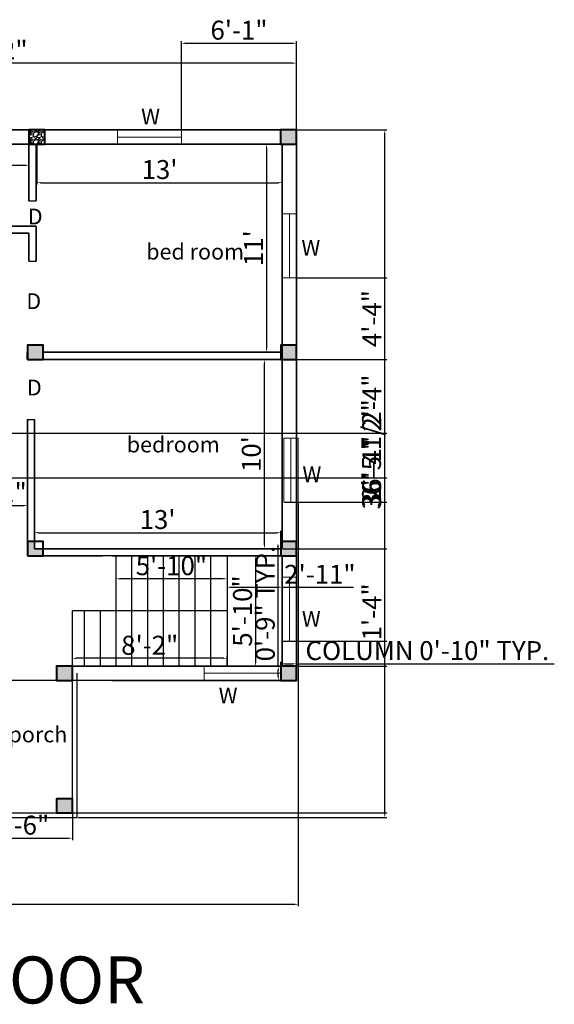
# Model space of a CAD drawing. Units: inches. Extents: x 1989 to 3287, y 1752 to 2384.
# Tile 5 of 5: x 2948 to 3287, y 1752 to 2377. Entities that reach past the tile are written whole.
import ezdxf

# ---------------------------------------------------------------- set-up
doc = ezdxf.new("R2010")
doc.units = ezdxf.units.IN
for name, color, linetype, lineweight in [('A-ANNO-DIMS', 2, 'Continuous', 18), ('A-ANNO-TEXT', 7, 'Continuous', 18), ('A-AREA-IDEN', 7, 'Continuous', 18), ('A-COLS', 1, 'Continuous', 40), ('A-COLS-PATT', 8, 'Continuous', 13), ('A-DOOR', 3, 'Continuous', 25), ('A-FLOR-EDGE', 7, 'Continuous', 25), ('A-FLOR-STRS', 7, 'Continuous', 25), ('A-GLAZ', 4, 'Continuous', 18), ('A-WALL', 7, 'Continuous', 35)]:
    doc.layers.add(name, color=color, linetype=linetype, lineweight=lineweight)
doc.styles.get("Standard").update_dxf_attribs({"font": 'arial.ttf'})
doc.dimstyles.new('ISO-25', dxfattribs={"dimtxt": 12, "dimasz": 2.5, "dimexe": 1.25, "dimexo": 0.625, "dimtad": 1, "dimdec": 0, "dimlunit": 4, "dimtxsty": 'Standard', "dimcen": 2.5, "dimadec": 0, "dimazin": 0, "dimtfac": 1, "dimtdec": 0, "dimtmove": 0, "dimatfit": 3, "dimfxl": 1, "dimarcsym": 0})

# ---------------------------------------------------------------- blocks, each defined once
blk = doc.blocks.new('*D19')
at = {"layer": 'A-ANNO-DIMS', "color": 0, "lineweight": -2, "transparency": 16777216}
for p, q in [((2915.71, 1873.05), (2915.71, 1856.37)), ((2981.21, 1873.05), (2981.21, 1856.37)), ((2918.21, 1857.62), (2978.71, 1857.62))]:
    blk.add_line(p, q, dxfattribs=at)
at = {"layer": 'A-ANNO-DIMS', "color": 0, "transparency": 16777216}
for points in [[(2918.21, 1858.04), (2918.21, 1857.2), (2915.71, 1857.62)], [(2978.71, 1858.04), (2978.71, 1857.2), (2981.21, 1857.62)]]:
    blk.add_solid(points, dxfattribs=at)
at = {"layer": 'Defpoints', "color": 0, "transparency": 16777216}
for p in [(2915.71, 1873.68), (2981.21, 1873.68), (2981.21, 1857.62)]:
    blk.add_point(p, dxfattribs=at)
at = {"layer": 'A-ANNO-DIMS', "color": 0, "transparency": 16777216, "insert": (2948.46, 1864.37), "char_height": 12, "attachment_point": 5}
blk.add_mtext('5\'-6"', dxfattribs=at)
blk = doc.blocks.new('*D20')
at = {"layer": 'A-ANNO-DIMS', "color": 0, "lineweight": -2, "transparency": 16777216}
for p, q in [((3079.21, 2028.42), (3079.21, 2015.48)), ((3114.21, 2028.42), (3114.21, 2015.48)), ((3081.71, 2016.73), (3111.71, 2016.73)), ((3114.21, 2016.73), (3159.39, 2016.73))]:
    blk.add_line(p, q, dxfattribs=at)
at = {"layer": 'A-ANNO-DIMS', "color": 0, "transparency": 16777216}
for points in [[(3081.71, 2017.15), (3081.71, 2016.31), (3079.21, 2016.73)], [(3111.71, 2017.15), (3111.71, 2016.31), (3114.21, 2016.73)]]:
    blk.add_solid(points, dxfattribs=at)
at = {"layer": 'Defpoints', "color": 0, "transparency": 16777216}
for p in [(3079.21, 2029.04), (3114.21, 2029.04), (3114.21, 2016.73)]:
    blk.add_point(p, dxfattribs=at)
at = {"layer": 'A-ANNO-DIMS', "color": 0, "transparency": 16777216, "insert": (3138.05, 2023.38), "char_height": 12, "attachment_point": 5}
blk.add_mtext('2\'-11"', dxfattribs=at)
blk = doc.blocks.new('*D21')
at = {"layer": 'A-ANNO-DIMS', "color": 0, "lineweight": -2, "transparency": 16777216}
for p, q in [((3079.83, 2036.68), (3098.58, 2036.68)), ((3097.33, 2034.18), (3097.33, 1969.18)), ((3079.83, 1966.68), (3098.58, 1966.68))]:
    blk.add_line(p, q, dxfattribs=at)
at = {"layer": 'A-ANNO-DIMS', "color": 0, "transparency": 16777216}
for points in [[(3096.91, 2034.18), (3097.75, 2034.18), (3097.33, 2036.68)], [(3096.91, 1969.18), (3097.75, 1969.18), (3097.33, 1966.68)]]:
    blk.add_solid(points, dxfattribs=at)
at = {"layer": 'Defpoints', "color": 0, "transparency": 16777216}
for p in [(3079.21, 2036.68), (3079.21, 1966.68), (3097.33, 1966.68)]:
    blk.add_point(p, dxfattribs=at)
at = {"layer": 'A-ANNO-DIMS', "color": 0, "transparency": 16777216, "insert": (3090.58, 2001.68), "char_height": 12, "attachment_point": 5, "rotation": 90}
blk.add_mtext('5\'-10"', dxfattribs=at)
blk = doc.blocks.new('*D22')
at = {"layer": 'A-ANNO-DIMS', "color": 0, "lineweight": -2, "transparency": 16777216}
for p, q in [((3008.71, 2036.05), (3008.71, 2020.84)), ((3079.21, 2036.05), (3079.21, 2020.84)), ((3076.71, 2022.09), (3011.21, 2022.09))]:
    blk.add_line(p, q, dxfattribs=at)
at = {"layer": 'A-ANNO-DIMS', "color": 0, "transparency": 16777216}
for points in [[(3011.21, 2022.5), (3011.21, 2021.67), (3008.71, 2022.09)], [(3076.71, 2022.5), (3076.71, 2021.67), (3079.21, 2022.09)]]:
    blk.add_solid(points, dxfattribs=at)
at = {"layer": 'Defpoints', "color": 0, "transparency": 16777216}
for p in [(3008.71, 2036.68), (3079.21, 2036.68), (3008.71, 2022.09)]:
    blk.add_point(p, dxfattribs=at)
at = {"layer": 'A-ANNO-DIMS', "color": 0, "transparency": 16777216, "insert": (3043.96, 2028.84), "char_height": 12, "attachment_point": 5}
blk.add_mtext('5\'-10"', dxfattribs=at)
blk = doc.blocks.new('*D23')
at = {"layer": 'A-ANNO-DIMS', "color": 0, "lineweight": -2, "transparency": 16777216}
for p, q in [((2981.21, 1967.3), (2981.21, 1972.92)), ((3079.21, 1967.3), (3079.21, 1972.92)), ((3076.71, 1971.67), (2983.71, 1971.67))]:
    blk.add_line(p, q, dxfattribs=at)
at = {"layer": 'A-ANNO-DIMS', "color": 0, "transparency": 16777216}
for points in [[(2983.71, 1972.08), (2983.71, 1971.25), (2981.21, 1971.67)], [(3076.71, 1972.08), (3076.71, 1971.25), (3079.21, 1971.67)]]:
    blk.add_solid(points, dxfattribs=at)
at = {"layer": 'Defpoints', "color": 0, "transparency": 16777216}
for p in [(2981.21, 1971.67), (2981.21, 1966.68), (3079.21, 1966.68)]:
    blk.add_point(p, dxfattribs=at)
at = {"layer": 'A-ANNO-DIMS', "color": 0, "transparency": 16777216, "insert": (3030.21, 1978.42), "char_height": 12, "attachment_point": 5}
blk.add_mtext('8\'-2"', dxfattribs=at)
blk = doc.blocks.new('*D27')
at = {"layer": 'A-ANNO-DIMS', "color": 0, "lineweight": -2, "transparency": 16777216}
for p, q in [((2737.21, 2307.3), (2737.21, 2350.26)), ((3120.71, 2349.01), (2739.71, 2349.01)), ((3123.21, 2307.3), (3123.21, 2350.26))]:
    blk.add_line(p, q, dxfattribs=at)
at = {"layer": 'A-ANNO-DIMS', "color": 0, "transparency": 16777216}
for points in [[(2739.71, 2349.43), (2739.71, 2348.6), (2737.21, 2349.01)], [(3120.71, 2349.43), (3120.71, 2348.6), (3123.21, 2349.01)]]:
    blk.add_solid(points, dxfattribs=at)
at = {"layer": 'Defpoints', "color": 0, "transparency": 16777216}
for p in [(2737.21, 2349.01), (2737.21, 2306.68), (3123.21, 2306.68)]:
    blk.add_point(p, dxfattribs=at)
at = {"layer": 'A-ANNO-DIMS', "color": 0, "transparency": 16777216, "insert": (2930.21, 2355.77), "char_height": 12, "attachment_point": 5}
blk.add_mtext('32\'-2"', dxfattribs=at)
blk = doc.blocks.new('*D28')
at = {"layer": 'A-ANNO-DIMS', "color": 0, "lineweight": -2, "transparency": 16777216}
for p, q in [((3113.58, 2297.68), (3102.92, 2297.68)), ((3104.17, 2295.18), (3104.17, 2168.18)), ((3113.58, 2165.68), (3102.92, 2165.68))]:
    blk.add_line(p, q, dxfattribs=at)
at = {"layer": 'A-ANNO-DIMS', "color": 0, "transparency": 16777216}
for points in [[(3103.76, 2295.18), (3104.59, 2295.18), (3104.17, 2297.68)], [(3103.76, 2168.18), (3104.59, 2168.18), (3104.17, 2165.68)]]:
    blk.add_solid(points, dxfattribs=at)
at = {"layer": 'Defpoints', "color": 0, "transparency": 16777216}
for p in [(3114.21, 2297.68), (3104.17, 2165.68), (3114.21, 2165.68)]:
    blk.add_point(p, dxfattribs=at)
at = {"layer": 'A-ANNO-DIMS', "color": 0, "transparency": 16777216, "insert": (3097.52, 2231.68), "char_height": 12, "attachment_point": 5, "rotation": 90}
blk.add_mtext("11'", dxfattribs=at)
blk = doc.blocks.new('*D29')
at = {"layer": 'A-ANNO-DIMS', "color": 0, "lineweight": -2, "transparency": 16777216}
for p, q in [((2958.71, 2297.05), (2958.71, 2271.98)), ((3114.21, 2297.05), (3114.21, 2271.98)), ((2961.21, 2273.23), (3111.71, 2273.23))]:
    blk.add_line(p, q, dxfattribs=at)
at = {"layer": 'A-ANNO-DIMS', "color": 0, "transparency": 16777216}
for points in [[(2961.21, 2273.65), (2961.21, 2272.82), (2958.71, 2273.23)], [(3111.71, 2273.65), (3111.71, 2272.82), (3114.21, 2273.23)]]:
    blk.add_solid(points, dxfattribs=at)
at = {"layer": 'Defpoints', "color": 0, "transparency": 16777216}
for p in [(2958.71, 2297.68), (3114.21, 2297.68), (3114.21, 2273.23)]:
    blk.add_point(p, dxfattribs=at)
at = {"layer": 'A-ANNO-DIMS', "color": 0, "transparency": 16777216, "insert": (3036.46, 2279.99), "char_height": 12, "attachment_point": 5}
blk.add_mtext("13'", dxfattribs=at)
blk = doc.blocks.new('*D39')
at = {"layer": 'A-ANNO-DIMS', "color": 0, "lineweight": -2, "transparency": 16777216}
for p, q in [((2883.71, 2297.05), (2883.71, 2282.99)), ((2953.71, 2297.05), (2953.71, 2282.99)), ((2886.21, 2284.24), (2951.21, 2284.24))]:
    blk.add_line(p, q, dxfattribs=at)
at = {"layer": 'A-ANNO-DIMS', "color": 0, "transparency": 16777216}
for points in [[(2886.21, 2284.65), (2886.21, 2283.82), (2883.71, 2284.24)], [(2951.21, 2284.65), (2951.21, 2283.82), (2953.71, 2284.24)]]:
    blk.add_solid(points, dxfattribs=at)
at = {"layer": 'Defpoints', "color": 0, "transparency": 16777216}
for p in [(2883.71, 2297.68), (2953.71, 2297.68), (2953.71, 2284.24)]:
    blk.add_point(p, dxfattribs=at)
at = {"layer": 'A-ANNO-DIMS', "color": 0, "transparency": 16777216, "insert": (2918.71, 2290.99), "char_height": 12, "attachment_point": 5}
blk.add_mtext('5\'-10"', dxfattribs=at)
blk = doc.blocks.new('*D42')
at = {"layer": 'A-ANNO-DIMS', "color": 0, "lineweight": -2, "transparency": 16777216}
for p, q in [((3113.58, 2161.18), (3101.67, 2161.18)), ((3102.92, 2043.68), (3102.92, 2158.68)), ((3113.58, 2041.18), (3101.67, 2041.18))]:
    blk.add_line(p, q, dxfattribs=at)
at = {"layer": 'A-ANNO-DIMS', "color": 0, "transparency": 16777216}
for points in [[(3102.51, 2158.68), (3103.34, 2158.68), (3102.92, 2161.18)], [(3102.51, 2043.68), (3103.34, 2043.68), (3102.92, 2041.18)]]:
    blk.add_solid(points, dxfattribs=at)
at = {"layer": 'Defpoints', "color": 0, "transparency": 16777216}
for p in [(3102.92, 2161.18), (3114.21, 2161.18), (3114.21, 2041.18)]:
    blk.add_point(p, dxfattribs=at)
at = {"layer": 'A-ANNO-DIMS', "color": 0, "transparency": 16777216, "insert": (3096.17, 2101.18), "char_height": 12, "attachment_point": 5, "rotation": 90}
blk.add_mtext("10'", dxfattribs=at)
blk = doc.blocks.new('*D43')
at = {"layer": 'A-ANNO-DIMS', "color": 0, "lineweight": -2, "transparency": 16777216}
for p, q in [((2957.21, 2041.8), (2957.21, 2052.59)), ((2959.71, 2051.34), (3110.71, 2051.34)), ((3113.21, 2041.8), (3113.21, 2052.59))]:
    blk.add_line(p, q, dxfattribs=at)
at = {"layer": 'A-ANNO-DIMS', "color": 0, "transparency": 16777216}
for points in [[(2959.71, 2051.76), (2959.71, 2050.92), (2957.21, 2051.34)], [(3110.71, 2051.76), (3110.71, 2050.92), (3113.21, 2051.34)]]:
    blk.add_solid(points, dxfattribs=at)
at = {"layer": 'Defpoints', "color": 0, "transparency": 16777216}
for p in [(3113.21, 2051.34), (2957.21, 2041.18), (3113.21, 2041.18)]:
    blk.add_point(p, dxfattribs=at)
at = {"layer": 'A-ANNO-DIMS', "color": 0, "transparency": 16777216, "insert": (3035.21, 2058.1), "char_height": 12, "attachment_point": 5}
blk.add_mtext("13'", dxfattribs=at)
blk = doc.blocks.new('*D47')
at = {"layer": 'A-ANNO-DIMS', "color": 0, "lineweight": -2, "transparency": 16777216}
for p, q in [((2915.71, 2037.3), (2915.71, 2069.77)), ((2918.21, 2068.52), (2950.21, 2068.52)), ((2952.71, 2037.3), (2952.71, 2069.77))]:
    blk.add_line(p, q, dxfattribs=at)
at = {"layer": 'A-ANNO-DIMS', "color": 0, "transparency": 16777216}
for points in [[(2918.21, 2068.93), (2918.21, 2068.1), (2915.71, 2068.52)], [(2950.21, 2068.93), (2950.21, 2068.1), (2952.71, 2068.52)]]:
    blk.add_solid(points, dxfattribs=at)
at = {"layer": 'Defpoints', "color": 0, "transparency": 16777216}
for p in [(2952.71, 2068.52), (2915.71, 2036.68), (2952.71, 2036.68)]:
    blk.add_point(p, dxfattribs=at)
at = {"layer": 'A-ANNO-DIMS', "color": 0, "transparency": 16777216, "insert": (2934.21, 2075.27), "char_height": 12, "attachment_point": 5}
blk.add_mtext('3\'-1"', dxfattribs=at)
blk = doc.blocks.new('WIN-EXT-STANDARD')
blk.add_line((4.5, 0), (4.5, 40.55))
blk.add_lwpolyline([(0, 40.55), (9, 40.55), (9, 0), (0, 0)], close=True)
blk = doc.blocks.new('WIN-STAIR-FRONT')
blk.add_line((0, 4.5), (48.49, 4.5))
blk.add_lwpolyline([(48.49, 9), (0, 9), (0, 0), (48.49, 0)], close=True)
blk = doc.blocks.new('COLUMN-10X9')
blk.add_lwpolyline([(0, 0), (10, 0), (10, 9), (0, 9)], close=True)
blk = doc.blocks.new('*D61')
at = {"layer": 'A-ANNO-DIMS', "color": 0, "lineweight": -2, "transparency": 16777216}
for p, q in [((3113.2, 1967.3), (3113.2, 1969.43)), ((3115.7, 1968.18), (3120.7, 1968.18)), ((3123.2, 1967.3), (3123.2, 1969.43)), ((3123.2, 1968.18), (3286.59, 1968.18))]:
    blk.add_line(p, q, dxfattribs=at)
at = {"layer": 'A-ANNO-DIMS', "color": 0, "transparency": 16777216}
for points in [[(3115.7, 1968.6), (3115.7, 1967.76), (3113.2, 1968.18)], [(3120.7, 1968.6), (3120.7, 1967.76), (3123.2, 1968.18)]]:
    blk.add_solid(points, dxfattribs=at)
at = {"layer": 'Defpoints', "color": 0, "transparency": 16777216}
for p in [(3113.2, 1966.68), (3123.2, 1968.18), (3123.2, 1966.68)]:
    blk.add_point(p, dxfattribs=at)
at = {"layer": 'A-ANNO-DIMS', "color": 0, "transparency": 16777216, "insert": (3206.14, 1975.01), "char_height": 12, "attachment_point": 5}
blk.add_mtext('COLUMN 0\'-10" TYP.', dxfattribs=at)
blk = doc.blocks.new('*D62')
at = {"layer": 'A-ANNO-DIMS', "color": 0, "lineweight": -2, "transparency": 16777216}
for p, q in [((3111.7, 1966.68), (3111.7, 2043.58)), ((3112.58, 1966.68), (3110.45, 1966.68)), ((3111.7, 1960.18), (3111.7, 1964.18)), ((3112.58, 1957.68), (3110.45, 1957.68))]:
    blk.add_line(p, q, dxfattribs=at)
at = {"layer": 'A-ANNO-DIMS', "color": 0, "transparency": 16777216}
for points in [[(3111.29, 1964.18), (3112.12, 1964.18), (3111.7, 1966.68)], [(3111.29, 1960.18), (3112.12, 1960.18), (3111.7, 1957.68)]]:
    blk.add_solid(points, dxfattribs=at)
at = {"layer": 'Defpoints', "color": 0, "transparency": 16777216}
for p in [(3111.7, 1966.68), (3113.2, 1966.68), (3113.2, 1957.68)]:
    blk.add_point(p, dxfattribs=at)
at = {"layer": 'A-ANNO-DIMS', "color": 0, "transparency": 16777216, "insert": (3104.95, 2006.38), "char_height": 12, "attachment_point": 5, "rotation": 90}
blk.add_mtext('0\'-9" TYP.', dxfattribs=at)
blk = doc.blocks.new('*D64')
at = {"layer": 'A-ANNO-DIMS', "color": 0, "lineweight": -2, "transparency": 16777216}
for p, q in [((2521.26, 2306.68), (3180.41, 2306.68)), ((3179.16, 1876.18), (3179.16, 2304.18)), ((2379.26, 1873.68), (3180.41, 1873.68))]:
    blk.add_line(p, q, dxfattribs=at)
at = {"layer": 'A-ANNO-DIMS', "color": 0, "transparency": 16777216}
for points in [[(3178.74, 2304.18), (3179.58, 2304.18), (3179.16, 2306.68)], [(3178.74, 1876.18), (3179.58, 1876.18), (3179.16, 1873.68)]]:
    blk.add_solid(points, dxfattribs=at)
at = {"layer": 'Defpoints', "color": 0, "transparency": 16777216}
for p in [(2520.64, 2306.68), (3179.16, 2306.68), (2378.64, 1873.68)]:
    blk.add_point(p, dxfattribs=at)
at = {"layer": 'A-ANNO-DIMS', "color": 0, "transparency": 16777216, "insert": (3172.4, 2090.18), "char_height": 12, "attachment_point": 5, "rotation": 90}
blk.add_mtext('36\'-1"', dxfattribs=at)
blk = doc.blocks.new('*D65')
at = {"layer": 'A-ANNO-DIMS', "color": 0, "lineweight": -2, "transparency": 16777216}
for p, q in [((3124.21, 2069.99), (3124.21, 1814.48)), ((2671.06, 1892.56), (2671.06, 1814.48)), ((2673.56, 1815.73), (3121.71, 1815.73))]:
    blk.add_line(p, q, dxfattribs=at)
at = {"layer": 'A-ANNO-DIMS', "color": 0, "transparency": 16777216}
for points in [[(2673.56, 1816.15), (2673.56, 1815.31), (2671.06, 1815.73)], [(3121.71, 1816.15), (3121.71, 1815.31), (3124.21, 1815.73)]]:
    blk.add_solid(points, dxfattribs=at)
at = {"layer": 'Defpoints', "color": 0, "transparency": 16777216}
for p in [(3124.21, 2070.62), (2671.06, 1893.19), (3124.21, 1815.73)]:
    blk.add_point(p, dxfattribs=at)
at = {"layer": 'A-ANNO-DIMS', "color": 0, "transparency": 16777216, "insert": (2897.63, 1822.49), "char_height": 12, "attachment_point": 5}
blk.add_mtext('37\'-9"', dxfattribs=at)
blk = doc.blocks.new('*D66')
at = {"layer": 'A-ANNO-DIMS', "color": 0, "lineweight": -2, "transparency": 16777216}
for p, q in [((3123.83, 2306.68), (3180.41, 2306.68)), ((3179.16, 1873.18), (3179.16, 2304.18)), ((2984.83, 1870.68), (3180.41, 1870.68))]:
    blk.add_line(p, q, dxfattribs=at)
at = {"layer": 'A-ANNO-DIMS', "color": 0, "transparency": 16777216}
for points in [[(3178.74, 2304.18), (3179.58, 2304.18), (3179.16, 2306.68)], [(3178.74, 1873.18), (3179.58, 1873.18), (3179.16, 1870.68)]]:
    blk.add_solid(points, dxfattribs=at)
at = {"layer": 'Defpoints', "color": 0, "transparency": 16777216}
for p in [(3123.21, 2306.68), (3179.16, 2306.68), (2984.21, 1870.68)]:
    blk.add_point(p, dxfattribs=at)
at = {"layer": 'A-ANNO-DIMS', "color": 0, "transparency": 16777216, "insert": (3172.4, 2088.68), "char_height": 12, "attachment_point": 5, "rotation": 90}
blk.add_mtext('36\'-4"', dxfattribs=at)
blk = doc.blocks.new('*D69')
at = {"layer": 'A-ANNO-DIMS', "color": 0, "lineweight": -2, "transparency": 16777216}
for p, q in [((3123.83, 2212.94), (3180.41, 2212.94)), ((3179.16, 2163.68), (3179.16, 2210.44)), ((3123.83, 2161.18), (3180.41, 2161.18))]:
    blk.add_line(p, q, dxfattribs=at)
at = {"layer": 'A-ANNO-DIMS', "color": 0, "transparency": 16777216}
for points in [[(3178.74, 2210.44), (3179.58, 2210.44), (3179.16, 2212.94)], [(3178.74, 2163.68), (3179.58, 2163.68), (3179.16, 2161.18)]]:
    blk.add_solid(points, dxfattribs=at)
at = {"layer": 'Defpoints', "color": 0, "transparency": 16777216}
for p in [(3123.21, 2212.94), (3179.16, 2212.94), (3123.21, 2161.18)]:
    blk.add_point(p, dxfattribs=at)
at = {"layer": 'A-ANNO-DIMS', "color": 0, "transparency": 16777216, "insert": (3172.53, 2187.06), "char_height": 12, "attachment_point": 5, "rotation": 90}
blk.add_mtext('4\'-4"', dxfattribs=at)
blk = doc.blocks.new('*D70')
at = {"layer": 'A-ANNO-DIMS', "color": 0, "lineweight": -2, "transparency": 16777216}
for p, q in [((3179.16, 2070.62), (3179.16, 2134.43)), ((3115.83, 2070.62), (3180.41, 2070.62)), ((3179.16, 2043.68), (3179.16, 2068.12)), ((3114.83, 2041.18), (3180.41, 2041.18))]:
    blk.add_line(p, q, dxfattribs=at)
at = {"layer": 'A-ANNO-DIMS', "color": 0, "transparency": 16777216}
for points in [[(3178.74, 2068.12), (3179.58, 2068.12), (3179.16, 2070.62)], [(3178.74, 2043.68), (3179.58, 2043.68), (3179.16, 2041.18)]]:
    blk.add_solid(points, dxfattribs=at)
at = {"layer": 'Defpoints', "color": 0, "transparency": 16777216}
for p in [(3115.21, 2070.62), (3179.16, 2070.62), (3114.21, 2041.18)]:
    blk.add_point(p, dxfattribs=at)
at = {"layer": 'A-ANNO-DIMS', "color": 0, "transparency": 16777216, "insert": (3172.33, 2103.78), "char_height": 12, "attachment_point": 5, "rotation": 90}
blk.add_mtext('2\'-5 1/2"', dxfattribs=at)
blk = doc.blocks.new('*D71')
at = {"layer": 'A-ANNO-DIMS', "color": 0, "lineweight": -2, "transparency": 16777216}
for p, q in [((3179.16, 1982.63), (3179.16, 2017.15)), ((3114.83, 1982.63), (3180.41, 1982.63)), ((3179.16, 1969.18), (3179.16, 1980.13)), ((3114.83, 1966.68), (3180.41, 1966.68))]:
    blk.add_line(p, q, dxfattribs=at)
at = {"layer": 'A-ANNO-DIMS', "color": 0, "transparency": 16777216}
for points in [[(3178.74, 1980.13), (3179.58, 1980.13), (3179.16, 1982.63)], [(3178.74, 1969.18), (3179.58, 1969.18), (3179.16, 1966.68)]]:
    blk.add_solid(points, dxfattribs=at)
at = {"layer": 'Defpoints', "color": 0, "transparency": 16777216}
for p in [(3114.21, 1982.63), (3179.16, 1982.63), (3114.21, 1966.68)]:
    blk.add_point(p, dxfattribs=at)
at = {"layer": 'A-ANNO-DIMS', "color": 0, "transparency": 16777216, "insert": (3172.51, 2001.14), "char_height": 12, "attachment_point": 5, "rotation": 90}
blk.add_mtext('1\'-4"', dxfattribs=at)
blk = doc.blocks.new('*D72')
at = {"layer": 'A-ANNO-DIMS', "color": 0, "lineweight": -2, "transparency": 16777216}
for p, q in [((3050.36, 2307.3), (3050.36, 2362.88)), ((3052.86, 2361.63), (3120.71, 2361.63)), ((3123.21, 2307.3), (3123.21, 2362.88))]:
    blk.add_line(p, q, dxfattribs=at)
at = {"layer": 'A-ANNO-DIMS', "color": 0, "transparency": 16777216}
for points in [[(3052.86, 2362.05), (3052.86, 2361.21), (3050.36, 2361.63)], [(3120.71, 2362.05), (3120.71, 2361.21), (3123.21, 2361.63)]]:
    blk.add_solid(points, dxfattribs=at)
at = {"layer": 'Defpoints', "color": 0, "transparency": 16777216}
for p in [(3123.21, 2361.63), (3050.36, 2306.68), (3123.21, 2306.68)]:
    blk.add_point(p, dxfattribs=at)
at = {"layer": 'A-ANNO-DIMS', "color": 0, "transparency": 16777216, "insert": (3086.79, 2368.38), "char_height": 12, "attachment_point": 5}
blk.add_mtext('6\'-1"', dxfattribs=at)
blk = doc.blocks.new('*D74')
at = {"layer": 'A-ANNO-DIMS', "color": 0, "lineweight": -2, "transparency": 16777216}
for p, q in [((3179.16, 2114.35), (3179.16, 2150.2)), ((2440.26, 2114.35), (3180.41, 2114.35)), ((3179.16, 2088.6), (3179.16, 2111.85)), ((2440.26, 2086.1), (3180.41, 2086.1))]:
    blk.add_line(p, q, dxfattribs=at)
at = {"layer": 'A-ANNO-DIMS', "color": 0, "transparency": 16777216}
for points in [[(3178.74, 2111.85), (3179.58, 2111.85), (3179.16, 2114.35)], [(3178.74, 2088.6), (3179.58, 2088.6), (3179.16, 2086.1)]]:
    blk.add_solid(points, dxfattribs=at)
at = {"layer": 'Defpoints', "color": 0, "transparency": 16777216}
for p in [(2439.64, 2114.35), (3179.16, 2114.35), (2439.64, 2086.1)]:
    blk.add_point(p, dxfattribs=at)
at = {"layer": 'A-ANNO-DIMS', "color": 0, "transparency": 16777216, "insert": (3172.51, 2133.53), "char_height": 12, "attachment_point": 5, "rotation": 90}
blk.add_mtext('2\'-4"', dxfattribs=at)

msp = doc.modelspace()

# ---------------------------------------------------------------- hatches: boundary and pattern name
at = {"layer": 'A-COLS-PATT'}
h = msp.add_hatch(dxfattribs=at)
h.set_pattern_fill('GRAVEL', color=256, scale=0.2)
h.paths.add_polyline_path([(3123.21, 2045.68), (3114.21, 2045.68), (3114.21, 2041.18), (3113.21, 2041.18), (3113.21, 2036.68), (3123.21, 2036.68)])
h.paths.add_polyline_path([(2962.75, 2170.18), (2952.75, 2170.18), (2952.75, 2161.18), (2962.75, 2161.18)])
h.paths.add_polyline_path([(2520.59, 2306.68), (2510.59, 2306.68), (2510.59, 2297.68), (2520.59, 2297.68)])
h.paths.add_polyline_path([(2520.64, 2170.18), (2511.64, 2170.18), (2511.64, 2161.18), (2520.64, 2161.18)])
h.paths.add_polyline_path([(2364.99, 2045.68), (2354.99, 2045.68), (2354.99, 2036.68), (2364.99, 2036.68)])
h.paths.add_polyline_path([(2361.14, 2170.18), (2351.14, 2170.18), (2351.14, 2161.18), (2361.14, 2161.18)])
h = msp.add_hatch(dxfattribs=at)
h.set_pattern_fill('GRAVEL', color=256, scale=0.2)
h.paths.add_polyline_path([(2963.71, 2306.68), (2953.71, 2306.68), (2953.71, 2297.68), (2963.71, 2297.68)])
h = msp.add_hatch(dxfattribs=at)
h.set_pattern_fill('GRAVEL', color=256, scale=0.2)
h.paths.add_polyline_path([(3123.17, 2306.68), (3113.17, 2306.68), (3113.17, 2297.68), (3123.17, 2297.68)])
h.paths.add_polyline_path([(3123.21, 2170.18), (3114.21, 2170.18), (3114.21, 2161.18), (3123.21, 2161.18)])
h = msp.add_hatch(dxfattribs=at)
h.set_pattern_fill('GRAVEL', color=256, scale=0.2)
h.paths.add_polyline_path([(2777.21, 2217.95), (2768.21, 2217.95), (2768.21, 2213.45), (2777.21, 2213.45)])
h.paths.add_polyline_path([(2915.71, 2217.95), (2911.21, 2217.95), (2911.21, 2213.45), (2915.71, 2213.45)])
h.paths.add_polyline_path([(2925.71, 1882.68), (2915.71, 1882.68), (2915.71, 1873.68), (2925.71, 1873.68)])
h.paths.add_polyline_path([(2981.21, 1882.68), (2971.21, 1882.68), (2971.21, 1873.68), (2981.21, 1873.68)])
h.paths.add_polyline_path([(2925.71, 1966.68), (2915.71, 1966.68), (2915.71, 1957.68), (2925.71, 1957.68)])
h.paths.add_polyline_path([(2981.21, 1966.68), (2971.21, 1966.68), (2971.21, 1957.68), (2981.21, 1957.68)])
h.paths.add_polyline_path([(3123.2, 1966.68), (3113.2, 1966.68), (3113.2, 1957.68), (3123.2, 1957.68)])
h.paths.add_polyline_path([(2962.71, 2041.18), (2957.21, 2041.18), (2957.21, 2045.68), (2952.71, 2045.68), (2952.71, 2036.68), (2962.71, 2036.68)])
h.paths.add_polyline_path([(3113.84, 2018.44), (3162.55, 2018.44), (3162.55, 2043.17), (3113.84, 2043.17)], flags=9)

# ---------------------------------------------------------------- linework, layer by layer
at = {"layer": 'A-COLS'}
for p, q in [((2952.71, 2161.18), (2952.71, 2165.68)), ((2981.21, 1966.68), (2971.21, 1966.68)), ((2971.21, 1966.68), (2971.21, 1957.68)), ((2981.21, 1882.68), (2971.21, 1882.68)), ((2971.21, 1882.68), (2971.21, 1873.68))]:
    msp.add_line(p, q, dxfattribs=at)
for points in [[(2953.71, 2297.68), (2963.71, 2297.68), (2963.71, 2306.68), (2953.71, 2306.68)], [(3113.17, 2297.68), (3123.17, 2297.68), (3123.17, 2306.68), (3113.17, 2306.68)], [(2952.75, 2161.18), (2962.75, 2161.18), (2962.75, 2170.18), (2952.75, 2170.18)], [(3113.22, 2161.18), (3123.22, 2161.18), (3123.22, 2170.18), (3113.22, 2170.18)], [(3113.21, 2036.68), (3123.21, 2036.68), (3123.21, 2045.68), (3113.21, 2045.68)], [(2971.21, 1957.68), (2981.21, 1957.68), (2981.21, 1966.68), (2971.21, 1966.68)], [(2971.21, 1873.68), (2981.21, 1873.68), (2981.21, 1882.68), (2971.21, 1882.68)]]:
    msp.add_lwpolyline(points, close=True, dxfattribs=at)
at = {"layer": 'A-DOOR'}
for p, q in [((2953.71, 2261.68), (2958.21, 2261.68)), ((2953.71, 2223.42), (2958.21, 2223.42))]:
    msp.add_line(p, q, dxfattribs=at)
for points in [[(2957.21, 2161.18), (2952.71, 2161.18)], [(2952.71, 2123.04), (2957.21, 2123.04)]]:
    msp.add_lwpolyline(points, dxfattribs=at)
at = {"layer": 'A-FLOR-EDGE'}
for p, q in [((2981.21, 1873.68), (2981.21, 1962.18)), ((2984.21, 1870.68), (2984.21, 1962.18)), ((3016.21, 1957.68), (2915.21, 1957.68)), ((2915.71, 1873.68), (2981.21, 1873.68)), ((2912.71, 1870.68), (2984.21, 1870.68))]:
    msp.add_line(p, q, dxfattribs=at)
at = {"layer": 'A-FLOR-STRS'}
for p, q in [((3079.21, 2036.68), (3000.21, 2036.68)), ((3008.71, 2036.68), (3008.71, 1966.68)), ((3018.71, 2036.68), (3018.71, 1966.68)), ((3028.71, 2036.68), (3028.71, 1966.68)), ((3038.71, 2036.68), (3038.71, 1966.68)), ((3048.71, 2036.68), (3048.71, 1966.68)), ((3058.71, 2036.68), (3058.71, 1966.68)), ((3068.71, 2036.68), (3068.71, 1966.68)), ((3079.21, 2036.68), (3079.21, 1966.68)), ((3079.21, 2001.68), (2981.21, 2001.68)), ((2981.21, 1966.68), (2981.21, 2001.68)), ((2988.71, 2001.68), (2988.71, 1966.68)), ((2998.71, 2001.68), (2998.71, 1966.68)), ((3079.21, 1966.68), (2981.21, 1966.68))]:
    msp.add_line(p, q, dxfattribs=at)
at = {"layer": 'A-WALL'}
for p, q in [((2953.71, 2297.68), (2913.71, 2297.68)), ((2953.71, 2297.68), (2953.71, 2261.68)), ((3114.21, 2297.68), (2958.21, 2297.68)), ((2958.21, 2297.68), (2958.21, 2261.68)), ((2883.71, 2241.18), (2953.71, 2241.18)), ((2913.71, 2245.68), (2958.21, 2245.68)), ((2953.71, 2241.18), (2953.71, 2223.42)), ((2958.21, 2245.68), (2958.21, 2235.48)), ((2958.21, 2236.79), (2958.21, 2223.42)), ((2952.71, 2165.68), (2952.75, 2165.68)), ((2953.71, 2161.18), (3114.21, 2161.18)), ((2962.75, 2165.68), (3114.21, 2165.68)), ((3114.21, 2161.18), (3114.21, 2041.18)), ((3123.21, 2161.18), (3123.21, 2036.68)), ((2952.71, 2036.68), (2952.71, 2123.04)), ((2957.21, 2041.18), (2957.21, 2123.04)), ((3000.21, 2036.68), (2952.71, 2036.68)), ((3113.21, 2041.18), (2957.21, 2041.18)), ((3037.71, 2041.18), (2967.56, 2041.18)), ((3016.21, 2036.68), (3006.21, 2036.68)), ((3006.21, 2036.68), (3006.21, 2036.68)), ((3016.21, 2036.68), (3067.05, 2036.68)), ((3114.21, 2036.68), (3037.71, 2036.68)), ((3114.21, 2041.18), (3042.21, 2041.18)), ((3114.21, 2036.68), (3079.21, 2036.68)), ((3114.21, 2036.68), (3114.21, 1966.68)), ((3123.21, 2036.68), (3123.21, 1957.68)), ((3006.21, 1966.68), (2971.21, 1966.68)), ((3114.21, 1966.68), (3016.21, 1966.68)), ((3123.21, 1957.68), (3006.21, 1957.68))]:
    msp.add_line(p, q, dxfattribs=at)
for points in [[(3123.21, 2090.68), (3123.21, 2306.68), (2737.21, 2306.68), (2737.21, 2137.49)], [(3114.21, 2099.68), (3114.21, 2297.68), (2746.21, 2297.68)], [(3016.21, 1966.68), (3006.21, 1966.68)], [(3006.21, 1957.68), (3016.21, 1957.68)]]:
    msp.add_lwpolyline(points, dxfattribs=at)

# ---------------------------------------------------------------- block references
at = {"layer": 'A-COLS'}
for p in [(2952.71, 2036.68), (3113.2, 1957.68)]:
    msp.add_blockref('COLUMN-10X9', p, dxfattribs=at)
at = {"layer": 'A-GLAZ', "rotation": 89.99999999999989}
msp.add_blockref('WIN-EXT-STANDARD', (3050.36, 2297.68), dxfattribs=at)
at = {"layer": 'A-GLAZ'}
for name, p in [('WIN-EXT-STANDARD', (3114.21, 2212.94)), ('WIN-EXT-STANDARD', (3115.21, 2070.62)), ('WIN-EXT-STANDARD', (3114.21, 1982.63)), ('WIN-STAIR-FRONT', (3064.71, 1957.68))]:
    msp.add_blockref(name, p, dxfattribs=at)

# ---------------------------------------------------------------- texts
at = {"layer": 'A-ANNO-TEXT', "attachment_point": 1}
for s, width, gutter_width, insert, char_height in [('W', 78.3523, 49.99, (3024.76, 2320.16), 10), ('D', 78.3523, 49.99, (2952.94, 2256.75), 10), ('W', 78.3523, 49.99, (3126.32, 2236.97), 10), ('D', 78.3523, 49.99, (2952.03, 2203.07), 10), ('D', 78.3523, 49.99, (2952.41, 2148.32), 10), ('W', 78.3523, 49.99, (3126.98, 2093.35), 10), ('W', 78.3523, 49.99, (3126.61, 2001.75), 10), ('W', 78.3523, 49.99, (3073.9, 1953.17), 10), ('FIRST FLOOR', 4273.6475, 149.09, (2778.54, 1782.67), 29.8187)]:
    msp.add_mtext_dynamic_manual_height_columns(s, width=width, gutter_width=gutter_width, heights=[0], dxfattribs=dict(at, insert=insert, char_height=char_height))
at = {"layer": 'A-AREA-IDEN', "char_height": 9.998, "attachment_point": 1}
for s, insert in [('bed room', (3028.01, 2234.52)), ('bedroom', (3015.69, 2112.23)), ('porch', (2940.73, 1928.41))]:
    msp.add_mtext_dynamic_manual_height_columns(s, width=78.3523, gutter_width=49.99, heights=[0], dxfattribs=dict(at, insert=insert))

# ---------------------------------------------------------------- dimensions: what is measured, and where the dimension line sits
at = {"layer": 'A-ANNO-DIMS'}
for base, p1, p2, override, picture, middle in [((3123.2091, 2361.63), (3050.3616, 2306.68), (3123.2091, 2306.68), {"dimdec": 1, "dimlfac": 1, "dimrnd": 0, "dimzin": 1, "dimdsep": 46, "dimlunit": 4, "dimfrac": 2}, '*D72', (3086.7853, 2368.3819)), ((2737.21, 2349.01), (3123.21, 2306.68), (2737.21, 2306.68), {"dimclrd": 0, "dimclre": 0, "dimclrt": 0}, '*D27', (2930.21, 2355.77)), ((2953.71, 2284.24), (2883.71, 2297.68), (2953.71, 2297.68), {"dimclrd": 0, "dimclre": 0, "dimclrt": 0}, '*D39', (2918.71, 2290.99)), ((3114.20906953, 2273.23166677), (2958.70906953, 2297.67998165), (3114.20906953, 2297.67998165), {"dimclrd": 0, "dimclre": 0, "dimclrt": 0}, '*D29', (3036.45906953, 2279.98763539)), ((2952.71, 2068.52), (2915.71, 2036.68), (2952.71, 2036.68), {"dimclrd": 0, "dimclre": 0, "dimclrt": 0}, '*D47', (2934.21, 2075.27)), ((3124.2091, 1815.73), (2671.0578, 1893.1857), (3124.2091, 2070.6179), {"dimdec": 1, "dimlfac": 1, "dimrnd": 0, "dimzin": 1, "dimdsep": 46, "dimlunit": 4, "dimfrac": 2}, '*D65', (2897.6335, 1822.486)), ((3113.21, 2051.34), (2957.21, 2041.18), (3113.21, 2041.18), {"dimclrd": 0, "dimclre": 0, "dimclrt": 0}, '*D43', (3035.21, 2058.1)), ((3008.7118, 2022.0856), (3079.2091, 2036.68), (3008.7118, 2036.68), {"dimclrd": 0, "dimclre": 0, "dimclrt": 0}, '*D22', (3043.9604, 2028.8375)), ((3114.21, 2016.73), (3079.21, 2029.04), (3114.21, 2029.04), {"dimclrd": 0, "dimclre": 0, "dimclrt": 0}, '*D20', (3138.05, 2023.38)), ((2981.21, 1971.67), (3079.21, 1966.68), (2981.21, 1966.68), {"dimclrd": 0, "dimclre": 0, "dimclrt": 0}, '*D23', (3030.21, 1978.42)), ((2981.20906953, 1857.62054686), (2915.70906953, 1873.67998165), (2981.20906953, 1873.67998165), {"dimclrd": 0, "dimclre": 0, "dimclrt": 0}, '*D19', (2948.45906953, 1864.37242271))]:
    dim = msp.add_linear_dim(base=base, p1=p1, p2=p2, dimstyle='ISO-25', override=override, dxfattribs=at)
    dim.commit()
    dim.dimension.update_dxf_attribs({"geometry": picture, "text_midpoint": middle})
for base, p1, p2, override, picture, middle in [((3179.16, 2306.68), (2378.64, 1873.68), (2520.64, 2306.68), {"dimdec": 1, "dimlfac": 1, "dimrnd": 0, "dimzin": 1, "dimdsep": 46, "dimlunit": 4, "dimfrac": 2}, '*D64', (3172.4, 2090.18)), ((3179.16, 2306.68), (2984.21, 1870.68), (3123.21, 2306.68), {"dimdec": 1, "dimlfac": 1, "dimrnd": 0, "dimzin": 1, "dimdsep": 46, "dimlunit": 4, "dimfrac": 2}, '*D66', (3172.4, 2088.68)), ((3104.17, 2165.68), (3114.21, 2297.68), (3114.21, 2165.68), {"dimclrd": 0, "dimclre": 0, "dimclrt": 0}, '*D28', (3097.52, 2231.68)), ((3179.16, 2212.94), (3123.21, 2161.18), (3123.21, 2212.94), {"dimdec": 1, "dimlfac": 1, "dimrnd": 0, "dimzin": 1, "dimdsep": 46, "dimlunit": 4, "dimfrac": 2}, '*D69', (3172.53, 2187.06)), ((3102.92, 2161.18), (3114.21, 2041.18), (3114.21, 2161.18), {"dimclrd": 0, "dimclre": 0, "dimclrt": 0}, '*D42', (3096.17, 2101.18)), ((3179.1591, 2114.3493), (2439.6365, 2086.1013), (2439.6365, 2114.3493), {"dimdec": 1, "dimlfac": 1, "dimrnd": 0, "dimzin": 1, "dimdsep": 46, "dimlunit": 4, "dimfrac": 2}, '*D74', (3172.5095, 2133.5261)), ((3179.16, 2070.62), (3114.21, 2041.18), (3115.21, 2070.62), {"dimdec": 1, "dimlfac": 1, "dimrnd": 0, "dimzin": 1, "dimdsep": 46, "dimlunit": 4, "dimfrac": 2}, '*D70', (3172.33, 2103.78)), ((3097.33, 1966.68), (3079.21, 2036.68), (3079.21, 1966.68), {"dimclrd": 0, "dimclre": 0, "dimclrt": 0}, '*D21', (3090.58, 2001.68)), ((3179.1591, 1982.6269), (3114.2091, 1966.68), (3114.2091, 1982.6269), {"dimdec": 1, "dimlfac": 1, "dimrnd": 0, "dimzin": 1, "dimdsep": 46, "dimlunit": 4, "dimfrac": 2}, '*D71', (3172.5095, 2001.1366))]:
    dim = msp.add_linear_dim(base=base, p1=p1, p2=p2, angle=90, dimstyle='ISO-25', override=override, dxfattribs=at)
    dim.commit()
    dim.dimension.update_dxf_attribs({"geometry": picture, "text_midpoint": middle})
dim = msp.add_linear_dim(base=(3111.7, 1966.68), p1=(3113.2, 1957.68), p2=(3113.2, 1966.68), angle=90, text='<> TYP.', dimstyle='ISO-25', override={"dimdec": 1, "dimlfac": 1, "dimrnd": 0, "dimzin": 1, "dimdsep": 46, "dimlunit": 4, "dimfrac": 2}, dxfattribs=at)
dim.commit()
dim.dimension.update_dxf_attribs({"geometry": '*D62', "text_midpoint": (3104.95, 2006.38)})
dim = msp.add_linear_dim(base=(3123.2, 1968.18), p1=(3113.2, 1966.68), p2=(3123.2, 1966.68), text='COLUMN <> TYP.', dimstyle='ISO-25', override={"dimdec": 1, "dimlfac": 1, "dimrnd": 0, "dimzin": 1, "dimdsep": 46, "dimlunit": 4, "dimfrac": 2}, dxfattribs=at)
dim.commit()
dim.dimension.update_dxf_attribs({"geometry": '*D61', "text_midpoint": (3206.14, 1975.01)})

doc.saveas('drawing.dxf')
